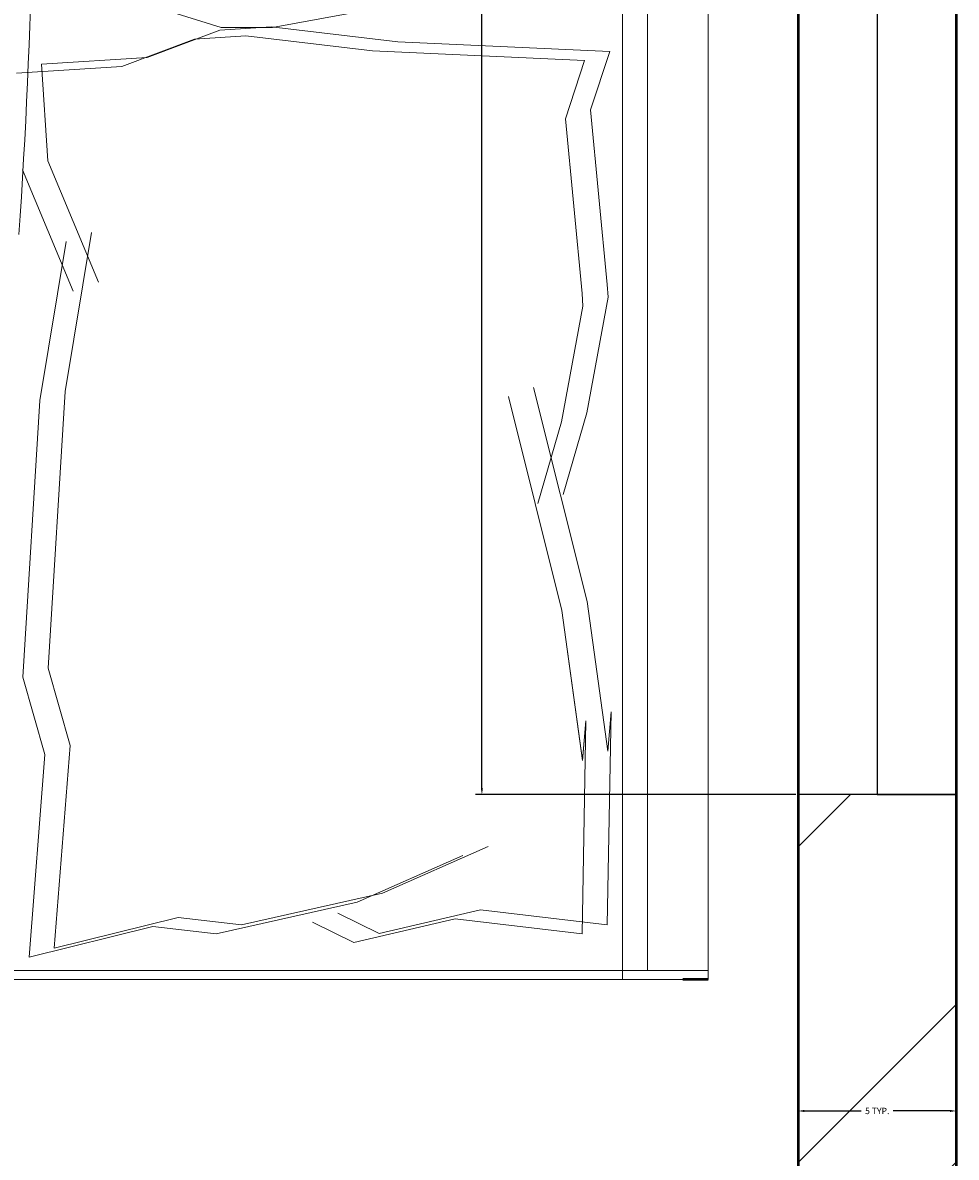
# Model space of a CAD drawing. Units: inches. Extents: x 1901 to 2863, y 888 to 2433.
# Tile 44 of 91: x 2726 to 2753, y 1563 to 1595. Entities that reach past the tile are written whole.
import ezdxf

# ---------------------------------------------------------------- set-up
doc = ezdxf.new("R2010")
doc.units = ezdxf.units.IN
for name, color, linetype, lineweight in [('A-ANNO-DIMS', 2, 'Continuous', 18), ('A-FURN', 8, 'Continuous', 18), ('A-GLAZ', 3, 'Continuous', 25), ('A-WALL', 7, 'Continuous', 50), ('A-WALL-PATT', 8, 'Continuous', 13)]:
    doc.layers.add(name, color=color, linetype=linetype, lineweight=lineweight)
doc.styles.get("Standard").update_dxf_attribs({"font": 'arial.ttf'})
doc.dimstyles.get("Standard").update_dxf_attribs({"dimtxt": 0.18, "dimasz": 0.18, "dimexe": 0.18, "dimexo": 0.0625, "dimgap": 0.09, "dimtad": 0, "dimtih": 1, "dimtoh": 1, "dimdec": 4, "dimzin": 0, "dimdsep": 46, "dimtxsty": 'Standard', "dimcen": 0.09, "dimadec": 0, "dimazin": 0, "dimtfac": 1, "dimtdec": 4, "dimtofl": 0, "dimtmove": 0, "dimatfit": 3, "dimfxl": 1, "dimtolj": 1, "dimtzin": 0, "dimarcsym": 0})

# ---------------------------------------------------------------- blocks, each defined once
blk = doc.blocks.new('BED-DOUBLE')
for p, q in [((0.026, 57.778), (0.026, 4.122)), ((0.744, 57.778), (30.62, 57.778)), ((0.744, 57.778), (30.62, 57.778)), ((18.633, 56.885), (15.109, 56.014)), ((18.633, 56.885), (15.109, 56.014)), ((19.351, 57.142), (15.827, 56.271)), ((19.351, 57.141), (15.827, 56.271)), ((18.18, 51.123), (18.633, 56.885)), ((18.18, 51.123), (18.633, 56.885)), ((18.898, 51.38), (19.351, 57.142)), ((18.898, 51.379), (19.351, 57.141)), ((7.22, 56.058), (10.106, 56.726)), ((7.22, 56.058), (10.106, 56.726)), ((10.106, 56.726), (11.28, 56.149)), ((10.106, 56.726), (11.28, 56.149)), ((2.897, 56.227), (2.788, 50.161)), ((2.897, 56.227), (2.788, 50.161)), ((2.897, 56.227), (6.502, 55.801)), ((2.897, 56.227), (6.502, 55.802)), ((3.615, 56.483), (3.506, 50.417)), ((3.615, 56.483), (3.506, 50.418)), ((3.615, 56.483), (7.22, 56.058)), ((3.615, 56.483), (7.22, 56.058)), ((6.502, 55.801), (9.388, 56.47)), ((6.502, 55.802), (9.388, 56.47)), ((13.307, 56.227), (9.297, 55.326)), ((13.307, 56.227), (9.297, 55.326)), ((9.388, 56.47), (10.563, 55.893)), ((9.388, 56.47), (10.563, 55.893)), ((14.025, 56.483), (10.015, 55.582)), ((14.025, 56.483), (10.015, 55.582)), ((15.109, 56.014), (13.307, 56.227)), ((15.109, 56.014), (13.307, 56.227)), ((15.827, 56.271), (14.025, 56.483)), ((15.827, 56.271), (14.025, 56.483)), ((10.015, 55.582), (7.007, 54.256)), ((10.015, 55.582), (7.007, 54.256)), ((9.297, 55.326), (6.289, 53.999)), ((9.297, 55.326), (6.289, 54)), ((3.506, 50.418), (3.598, 51.544)), ((3.506, 50.417), (3.598, 51.543)), ((3.598, 51.544), (4.19, 47.279)), ((3.598, 51.543), (4.19, 47.279)), ((19.523, 49.179), (18.898, 51.38)), ((19.523, 49.179), (18.898, 51.379)), ((2.788, 50.161), (2.881, 51.287)), ((2.788, 50.161), (2.881, 51.287)), ((2.881, 51.287), (3.472, 47.023)), ((2.881, 51.287), (3.472, 47.023)), ((18.806, 48.922), (18.18, 51.123)), ((18.806, 48.922), (18.18, 51.123)), ((19.039, 41.308), (19.523, 49.179)), ((19.039, 41.308), (19.523, 49.179)), ((18.322, 41.052), (18.806, 48.922)), ((18.322, 41.052), (18.806, 48.922)), ((4.19, 47.279), (5.709, 41.195)), ((4.19, 47.279), (5.709, 41.195)), ((3.472, 47.023), (4.991, 40.938)), ((3.472, 47.023), (4.991, 40.938)), ((4.869, 44.232), (4.2, 41.913)), ((4.869, 44.232), (4.2, 41.914)), ((4.151, 43.976), (3.482, 41.657)), ((4.151, 43.975), (3.482, 41.657)), ((3.482, 41.657), (2.875, 38.367)), ((3.482, 41.657), (2.875, 38.367)), ((4.2, 41.914), (3.593, 38.623)), ((4.2, 41.913), (3.593, 38.623)), ((17.573, 36.525), (18.322, 41.052)), ((17.573, 36.525), (18.322, 41.052)), ((18.291, 36.782), (19.039, 41.308)), ((18.291, 36.781), (19.039, 41.308)), ((3.593, 38.623), (3.615, 38.263)), ((3.593, 38.623), (3.615, 38.263)), ((2.875, 38.367), (2.897, 38.006)), ((2.875, 38.367), (2.897, 38.007)), ((3.615, 38.263), (4.088, 33.291)), ((3.615, 38.263), (4.088, 33.291)), ((19.538, 34.745), (18.096, 38.192)), ((19.538, 34.745), (18.096, 38.192)), ((2.897, 38.007), (3.371, 33.035)), ((2.897, 38.006), (3.371, 33.035)), ((18.82, 34.489), (17.378, 37.936)), ((18.82, 34.488), (17.378, 37.936)), ((18.993, 31.735), (18.82, 34.489)), ((18.993, 31.734), (18.82, 34.488)), ((4.088, 33.291), (3.542, 31.631)), ((4.088, 33.291), (3.542, 31.631)), ((3.371, 33.035), (2.824, 31.374)), ((3.371, 33.035), (2.824, 31.375)), ((16.706, 31.803), (19.71, 31.991)), ((16.706, 31.803), (19.71, 31.991)), ((14.64, 31.024), (16.706, 31.803)), ((14.64, 31.024), (16.706, 31.803)), ((15.988, 31.547), (18.993, 31.735)), ((15.988, 31.547), (18.993, 31.734)), ((2.824, 31.375), (8.859, 31.101)), ((2.824, 31.374), (8.859, 31.101)), ((3.542, 31.631), (9.577, 31.358)), ((3.542, 31.631), (9.577, 31.358)), ((9.577, 31.358), (13.182, 30.933)), ((9.577, 31.358), (13.182, 30.932)), ((13.922, 30.767), (15.988, 31.547)), ((13.922, 30.767), (15.988, 31.547)), ((8.859, 31.101), (12.464, 30.676)), ((8.859, 31.101), (12.464, 30.676)), ((13.182, 30.932), (14.64, 31.024)), ((13.182, 30.933), (14.64, 31.024)), ((8.85, 30.041), (12.422, 30.69)), ((8.85, 30.041), (12.422, 30.69)), ((12.422, 30.69), (13.883, 30.69)), ((12.422, 30.69), (13.883, 30.69)), ((12.464, 30.676), (13.922, 30.767)), ((12.464, 30.676), (13.922, 30.767)), ((13.883, 30.69), (15.993, 30.041)), ((13.883, 30.69), (15.993, 30.041))]:
    blk.add_line(p, q)
blk.add_arc((204.426, 23.944), 185.219, 176.08655, 186.78213)
blk.add_arc((204.426, 23.944), 185.219, 176.08655, 186.78213)
blk = doc.blocks.new('WIN-60')
for p, q in [((60, 2.25), (60, 4.5)), ((60, 4.5), (60, 0)), ((0, 2.25), (60, 2.25))]:
    blk.add_line(p, q)
blk = doc.blocks.new('*D19')
at = {"layer": 'A-ANNO-DIMS', "color": 0, "lineweight": -2, "transparency": 16777216}
for p, q in [((2748.364, 1633.499), (2739.246, 1633.499)), ((2739.426, 1633.319), (2739.426, 1603.682)), ((2739.426, 1573.679), (2739.426, 1603.316)), ((2748.364, 1573.499), (2739.246, 1573.499))]:
    blk.add_line(p, q, dxfattribs=at)
at = {"layer": 'A-ANNO-DIMS', "color": 0, "transparency": 16777216}
for points in [[(2739.396, 1633.319), (2739.456, 1633.319), (2739.426, 1633.499)], [(2739.396, 1573.679), (2739.456, 1573.679), (2739.426, 1573.499)]]:
    blk.add_solid(points, dxfattribs=at)
at = {"layer": 'Defpoints', "color": 0, "transparency": 16777216}
for p in [(2748.426, 1633.499), (2739.426, 1573.499), (2748.426, 1573.499)]:
    blk.add_point(p, dxfattribs=at)
at = {"layer": 'A-ANNO-DIMS', "color": 0, "transparency": 16777216, "insert": (2739.426, 1603.499), "char_height": 0.18, "attachment_point": 5}
blk.add_mtext('\\A1;WINDOW W1 60 TYP.', dxfattribs=at)
blk = doc.blocks.new('*D20')
at = {"layer": 'A-ANNO-DIMS', "color": 0, "lineweight": -2, "transparency": 16777216}
for p, q in [((2748.426, 1573.437), (2748.426, 1564.319)), ((2752.926, 1573.437), (2752.926, 1564.319)), ((2748.606, 1564.499), (2750.218, 1564.499)), ((2752.746, 1564.499), (2751.134, 1564.499))]:
    blk.add_line(p, q, dxfattribs=at)
at = {"layer": 'A-ANNO-DIMS', "color": 0, "transparency": 16777216}
for points in [[(2748.606, 1564.529), (2748.606, 1564.469), (2748.426, 1564.499)], [(2752.746, 1564.529), (2752.746, 1564.469), (2752.926, 1564.499)]]:
    blk.add_solid(points, dxfattribs=at)
at = {"layer": 'Defpoints', "color": 0, "transparency": 16777216}
for p in [(2748.426, 1573.499), (2752.926, 1573.499), (2752.926, 1564.499)]:
    blk.add_point(p, dxfattribs=at)
at = {"layer": 'A-ANNO-DIMS', "color": 0, "transparency": 16777216, "insert": (2750.676, 1564.499), "char_height": 0.18, "attachment_point": 5}
blk.add_mtext('\\A1;5 TYP.', dxfattribs=at)

msp = doc.modelspace()

# ---------------------------------------------------------------- hatches: boundary and pattern name
at = {"layer": 'A-WALL-PATT'}
h = msp.add_hatch(dxfattribs=at)
h.set_pattern_fill('ANSI32', color=256)
h.paths.add_polyline_path([(2443.926, 2139.888), (2439.426, 2139.888), (2439.426, 2069.348), (2441.676, 2069.348), (2443.926, 2069.348), (2443.926, 2078.634), (2521.926, 2078.634), (2521.926, 2075.067), (2524.176, 2075.067), (2526.426, 2075.067), (2526.426, 2078.634), (2571.755, 2078.634), (2571.755, 2080.884), (2571.755, 2083.134), (2443.926, 2083.134)])
h.paths.add_polyline_path([(2526.426, 2054.634), (2524.176, 2054.634), (2521.926, 2054.634), (2521.926, 2030.634), (2443.926, 2030.634), (2443.926, 2045.348), (2439.426, 2045.348), (2439.426, 1983.867), (2443.926, 1983.867), (2443.926, 2026.134), (2521.926, 2026.134), (2526.426, 2026.134)])
h.paths.add_polyline_path([(2443.926, 1923.867), (2439.426, 1923.867), (2439.426, 1872.634), (2443.926, 1872.634)])
h.paths.add_polyline_path([(2636.233, 1766.134), (2609.926, 1766.134), (2609.926, 1779.785), (2605.426, 1779.785), (2605.426, 1766.134), (2486.614, 1766.134), (2486.614, 1770.671), (2482.114, 1770.671), (2482.114, 1766.134), (2482.114, 1761.634), (2636.233, 1761.634), (2636.233, 1763.884)])
h.paths.add_polyline_path([(2519.536, 1663.384), (2519.536, 1665.634), (2494.926, 1665.634), (2481.831, 1665.634), (2481.831, 1663.384), (2481.831, 1661.134), (2490.426, 1661.134), (2490.426, 1640.157), (2494.926, 1640.157), (2494.926, 1661.134), (2519.536, 1661.134)])
h.paths.add_polyline_path([(2443.926, 1712.134), (2443.926, 1716.634), (2414.464, 1716.634), (2414.464, 1712.134), (2439.426, 1712.134), (2439.426, 1545.507), (2443.926, 1545.507), (2443.926, 1661.134), (2448.475, 1661.134), (2448.475, 1665.634), (2443.926, 1665.634)])
h.paths.add_polyline_path([(2343.426, 1712.134), (2365.525, 1712.134), (2365.525, 1714.384), (2365.525, 1716.634), (2333.871, 1716.634), (2333.871, 1714.384), (2333.871, 1712.134), (2338.926, 1712.134), (2338.926, 1575.634), (2338.926, 1545.507), (2343.426, 1545.507), (2343.426, 1547.507), (2343.426, 1580.134)])
h.paths.add_polyline_path([(2752.926, 1665.634), (2579.536, 1665.634), (2579.536, 1661.134), (2615.926, 1661.134), (2615.926, 1529.134), (2598.931, 1529.134), (2598.931, 1524.634), (2623.127, 1524.634), (2623.127, 1526.884), (2623.127, 1529.134), (2620.426, 1529.134), (2620.426, 1661.134), (2748.426, 1661.134), (2748.426, 1633.499), (2752.926, 1633.499)])
h.paths.add_polyline_path([(2752.926, 1419.929), (2748.426, 1419.929), (2748.426, 1400.134), (2659.426, 1400.134), (2659.426, 1444.333), (2657.176, 1444.333), (2654.926, 1444.333), (2654.926, 1400.134), (2643.649, 1400.134), (2643.649, 1395.634), (2748.426, 1395.634), (2748.426, 1364.035), (2752.926, 1364.035)])
h.paths.add_polyline_path([(2752.926, 1492.878), (2748.426, 1492.878), (2748.426, 1476.634), (2667.426, 1476.634), (2667.426, 1479.71), (2665.176, 1479.71), (2662.926, 1479.71), (2662.926, 1476.634), (2654.926, 1476.634), (2654.926, 1469.536), (2659.426, 1469.536), (2659.426, 1472.134), (2748.426, 1472.134), (2748.426, 1455.929), (2752.926, 1455.929)])
h.paths.add_polyline_path([(2752.926, 1304.035), (2748.426, 1304.035), (2748.426, 1263.634), (2738.66, 1263.634), (2738.66, 1259.134), (2752.926, 1259.134)])
h.paths.add_polyline_path([(2685.926, 1259.134), (2695.49, 1259.134), (2695.49, 1261.384), (2695.49, 1263.634), (2677.837, 1263.634), (2677.837, 1261.384), (2677.837, 1259.134), (2681.426, 1259.134), (2681.426, 1203.634), (2653.277, 1203.634), (2653.277, 1199.134), (2685.926, 1199.134), (2685.926, 1203.634)])
h.paths.add_polyline_path([(2609.426, 1395.634), (2611.848, 1395.634), (2611.848, 1400.134), (2598.888, 1400.134), (2598.888, 1397.884), (2598.888, 1395.634), (2604.926, 1395.634), (2604.926, 1268.134), (2554.726, 1268.134), (2554.726, 1265.884), (2554.726, 1263.634), (2604.926, 1263.634), (2604.926, 1203.634), (2571.306, 1203.634), (2571.306, 1199.134), (2604.926, 1199.134), (2629.277, 1199.134), (2629.277, 1201.384), (2629.277, 1203.634), (2609.426, 1203.634), (2609.426, 1258.634), (2609.426, 1259.134), (2654.804, 1259.134), (2654.804, 1263.634), (2609.426, 1263.634)])
h.paths.add_polyline_path([(2443.926, 1304.035), (2439.426, 1304.035), (2439.426, 1259.134), (2443.926, 1259.134), (2456.16, 1259.134), (2456.16, 1261.384), (2456.16, 1263.634), (2443.926, 1263.634)])
h.paths.add_polyline_path([(2525.426, 1263.634), (2531.778, 1263.634), (2531.778, 1268.134), (2520.926, 1268.134), (2520.926, 1263.634), (2511.409, 1263.634), (2511.409, 1259.134), (2520.926, 1259.134), (2520.926, 1199.134), (2547.306, 1199.134), (2547.306, 1201.384), (2547.306, 1203.634), (2525.426, 1203.634)])
h.paths.add_polyline_path([(2443.926, 1434.842), (2439.426, 1434.842), (2439.426, 1364.035), (2441.676, 1364.035), (2443.926, 1364.035)])
h.paths.add_polyline_path([(2567.134, 1400.134), (2443.926, 1400.134), (2443.926, 1395.634), (2567.134, 1395.634)])
h.paths.add_polyline_path([(2443.926, 1545.507), (2439.426, 1545.507), (2439.426, 1494.842), (2443.926, 1494.842)])
h.paths.add_polyline_path([(2494.926, 1553.349), (2492.676, 1553.349), (2490.426, 1553.349), (2490.426, 1524.634), (2494.926, 1524.634), (2525.936, 1524.634), (2525.936, 1526.884), (2525.936, 1529.134), (2494.926, 1529.134)])
h.paths.add_polyline_path([(2752.926, 1573.499), (2748.426, 1573.499), (2748.426, 1529.134), (2657.759, 1529.134), (2657.759, 1524.634), (2662.926, 1524.634), (2662.926, 1498.631), (2667.426, 1498.631), (2667.426, 1524.634), (2748.426, 1524.634), (2748.426, 1516.878), (2752.926, 1516.878)])
h.paths.add_polyline_path([(2038.602, 2237.418), (2080.174, 2237.418), (2080.174, 2256.075), (2038.602, 2256.075)], flags=9)
h.paths.add_polyline_path([(2292.009, 1062.394), (2539.932, 1062.394), (2539.932, 1099.487), (2292.009, 1099.487)], flags=9)
h.paths.add_polyline_path([(2424.91, 1832.253), (2448.513, 1832.253), (2448.513, 1846.678), (2424.91, 1846.678)], flags=9)
h.paths.add_polyline_path([(2359.076, 1832.253), (2382.678, 1832.253), (2382.678, 1846.678), (2359.076, 1846.678)], flags=9)
h.paths.add_polyline_path([(2352.899, 1684.802), (2367.543, 1684.802), (2367.543, 1697.167), (2352.899, 1697.167)], flags=9)
h.paths.add_polyline_path([(2079.288, 1755.826), (2169.024, 1755.826), (2169.024, 1774.372), (2079.288, 1774.372)], flags=9)
h.paths.add_polyline_path([(2404.09, 1373.857), (2404.09, 1463.593), (2385.544, 1463.593), (2385.544, 1373.857)], flags=9)
h.paths.add_polyline_path([(2268.091, 2236.371), (2309.636, 2236.371), (2309.636, 2255.028), (2268.091, 2255.028)], flags=9)
h.paths.add_polyline_path([(2575.96, 1700.951), (2665.696, 1700.951), (2665.696, 1719.498), (2575.96, 1719.498)], flags=9)
h.paths.add_polyline_path([(2302.962, 1878.474), (2329.524, 1878.474), (2329.524, 1888.777), (2302.962, 1888.777)], flags=9)
h.paths.add_polyline_path([(2097.415, 2240.576), (2126.573, 2240.576), (2126.573, 2259.233), (2097.415, 2259.233)], flags=9)
h.paths.add_polyline_path([(2208.725, 2246.124), (2237.882, 2246.124), (2237.882, 2264.781), (2208.725, 2264.781)], flags=9)
h.paths.add_polyline_path([(2038.147, 1925.958), (2076.987, 1925.958), (2076.987, 1944.615), (2038.147, 1944.615)], flags=9)
h.paths.add_polyline_path([(2239.144, 1926.672), (2288.465, 1926.672), (2288.465, 1945.329), (2239.144, 1945.329)], flags=9)
h.paths.add_polyline_path([(2175.429, 2007.33), (2212.356, 2007.33), (2212.356, 2025.987), (2175.429, 2025.987)], flags=9)
h.paths.add_polyline_path([(2225.034, 2091.794), (2263.875, 2091.794), (2263.875, 2110.451), (2225.034, 2110.451)], flags=9)
h.paths.add_polyline_path([(2035.398, 2098.478), (2074.238, 2098.478), (2074.238, 2117.135), (2035.398, 2117.135)], flags=9)
h.paths.add_polyline_path([(2050.102, 2029.209), (2083.26, 2029.209), (2083.26, 2047.866), (2050.102, 2047.866)], flags=9)
h.paths.add_polyline_path([(2069.677, 1956.719), (2098.835, 1956.719), (2098.835, 1975.376), (2069.677, 1975.376)], flags=9)
h.paths.add_polyline_path([(2328.62, 1753.336), (2361.663, 1753.336), (2361.663, 1771.993), (2328.62, 1771.993)], flags=9)
h.paths.add_polyline_path([(2395.162, 2060.888), (2395.162, 2140.654), (2378.676, 2140.654), (2378.676, 2060.888)], flags=9)
h.paths.add_polyline_path([(2463.728, 2059.02), (2492.886, 2059.02), (2492.886, 2077.677), (2463.728, 2077.677)], flags=9)
h.paths.add_polyline_path([(2458.027, 2181.536), (2496.868, 2181.536), (2496.868, 2200.194), (2458.027, 2200.194)], flags=9)
h.paths.add_polyline_path([(2456.855, 2228.831), (2498.401, 2228.831), (2498.401, 2247.488), (2456.855, 2247.488)], flags=9)
h.paths.add_polyline_path([(2527.577, 2243.074), (2556.735, 2243.074), (2556.735, 2261.731), (2527.577, 2261.731)], flags=9)
h.paths.add_polyline_path([(2694.461, 2232.767), (2736.033, 2232.767), (2736.033, 2251.425), (2694.461, 2251.425)], flags=9)
h.paths.add_polyline_path([(2637.821, 2249.225), (2666.979, 2249.225), (2666.979, 2267.882), (2637.821, 2267.882)], flags=9)
h.paths.add_polyline_path([(2623.687, 2183.541), (2662.528, 2183.541), (2662.528, 2202.199), (2623.687, 2202.199)], flags=9)
h.paths.add_polyline_path([(2691.965, 2021.5), (2725.124, 2021.5), (2725.124, 2040.157), (2691.965, 2040.157)], flags=9)
h.paths.add_polyline_path([(2621.043, 1975.912), (2662.335, 1975.912), (2662.335, 1994.569), (2621.043, 1994.569)], flags=9)
h.paths.add_polyline_path([(2479.032, 1927.62), (2519.844, 1927.62), (2519.844, 1946.277), (2479.032, 1946.277)], flags=9)
h.paths.add_polyline_path([(2670.941, 1849.076), (2716.005, 1849.076), (2716.005, 1867.734), (2670.941, 1867.734)], flags=9)
h.paths.add_polyline_path([(2523.613, 1782.956), (2550.175, 1782.956), (2550.175, 1793.26), (2523.613, 1793.26)], flags=9)
h.paths.add_polyline_path([(2450.841, 1207.331), (2492.386, 1207.331), (2492.386, 1225.989), (2450.841, 1225.989)], flags=9)
h.paths.add_polyline_path([(2527.751, 1203.841), (2556.908, 1203.841), (2556.908, 1222.499), (2527.751, 1222.499)], flags=9)
h.paths.add_polyline_path([(2639.111, 1207.2), (2668.268, 1207.2), (2668.268, 1225.857), (2639.111, 1225.857)], flags=9)
h.paths.add_polyline_path([(2692.594, 1218.965), (2734.167, 1218.965), (2734.167, 1237.623), (2692.594, 1237.623)], flags=9)
h.paths.add_polyline_path([(2669.266, 1366.329), (2708.106, 1366.329), (2708.106, 1384.987), (2669.266, 1384.987)], flags=25)
h.paths.add_polyline_path([(2463.313, 1358.031), (2502.153, 1358.031), (2502.153, 1376.688), (2463.313, 1376.688)], flags=9)
h.paths.add_polyline_path([(2494.725, 1449.963), (2531.652, 1449.963), (2531.652, 1468.62), (2494.725, 1468.62)], flags=9)
h.paths.add_polyline_path([(2675.565, 1422.157), (2708.724, 1422.157), (2708.724, 1440.815), (2675.565, 1440.815)], flags=25)
h.paths.add_polyline_path([(2685.634, 1493.891), (2714.792, 1493.891), (2714.792, 1512.548), (2685.634, 1512.548)], flags=9)
h.paths.add_polyline_path([(2686.805, 1529.913), (2725.645, 1529.913), (2725.645, 1548.57), (2686.805, 1548.57)], flags=25)
h.paths.add_polyline_path([(2503.651, 1537.991), (2552.972, 1537.991), (2552.972, 1556.648), (2503.651, 1556.648)], flags=9)
h.paths.add_polyline_path([(2291.713, 1643.504), (2318.275, 1643.504), (2318.275, 1653.807), (2291.713, 1653.807)], flags=9)
h.paths.add_polyline_path([(2450.626, 1610.52), (2477.189, 1610.52), (2477.189, 1620.824), (2450.626, 1620.824)], flags=9)
h.paths.add_polyline_path([(2359.985, 1551.814), (2422.253, 1551.814), (2422.253, 1562.117), (2359.985, 1562.117)], flags=9)
h.paths.add_polyline_path([(2280.106, 1249.006), (2321.651, 1249.006), (2321.651, 1267.663), (2280.106, 1267.663)], flags=9)
h.paths.add_polyline_path([(2164.057, 1274.232), (2193.215, 1274.232), (2193.215, 1292.889), (2164.057, 1292.889)], flags=9)
h.paths.add_polyline_path([(2118.21, 1277.694), (2151.252, 1277.694), (2151.252, 1296.351), (2118.21, 1296.351)], flags=9)
h.paths.add_polyline_path([(2031.946, 1268.529), (2073.519, 1268.529), (2073.519, 1287.187), (2031.946, 1287.187)], flags=9)
h.paths.add_polyline_path([(2050.199, 1409.079), (2089.04, 1409.079), (2089.04, 1427.736), (2050.199, 1427.736)], flags=9)
h.paths.add_polyline_path([(2243.743, 1421.032), (2282.584, 1421.032), (2282.584, 1439.689), (2243.743, 1439.689)], flags=9)
h.paths.add_polyline_path([(2190.746, 1509.769), (2231.558, 1509.769), (2231.558, 1528.426), (2190.746, 1528.426)], flags=9)
h.paths.add_polyline_path([(2058.392, 1475.415), (2091.55, 1475.415), (2091.55, 1494.073), (2058.392, 1494.073)], flags=9)
h.paths.add_polyline_path([(2062.447, 1553.09), (2091.605, 1553.09), (2091.605, 1571.747), (2062.447, 1571.747)], flags=9)
h.paths.add_polyline_path([(2219.524, 1590.365), (2266.147, 1590.365), (2266.147, 1609.022), (2219.524, 1609.022)], flags=9)
h.paths.add_polyline_path([(2041.072, 1584.188), (2079.912, 1584.188), (2079.912, 1602.845), (2041.072, 1602.845)], flags=9)

# ---------------------------------------------------------------- linework, layer by layer
at = {"layer": 'A-FURN'}
for p, q in [((2744.142, 1622.154), (2744.142, 1568.498)), ((2744.142, 1622.154), (2744.142, 1568.498)), ((2743.424, 1621.898), (2743.424, 1568.241)), ((2743.424, 1621.898), (2743.424, 1568.241)), ((2745.864, 1568.498), (2715.987, 1568.498)), ((2745.864, 1568.498), (2715.987, 1568.498))]:
    msp.add_line(p, q, dxfattribs=at)
at = {"layer": 'A-WALL'}
for p, q in [((2752.926, 1665.634), (2752.926, 1259.134)), ((2748.426, 1661.134), (2748.426, 1529.134)), ((2745.864, 1568.241), (2745.146, 1568.241))]:
    msp.add_line(p, q, dxfattribs=at)

# ---------------------------------------------------------------- block references
at = {"layer": 'A-FURN', "rotation": 180}
msp.add_blockref('BED-DOUBLE', (2745.89, 1626.019), dxfattribs=at)
at = {"layer": 'A-GLAZ', "rotation": 270.0000000000013}
msp.add_blockref('WIN-60', (2748.426, 1633.5), dxfattribs=at)

# ---------------------------------------------------------------- dimensions: what is measured, and where the dimension line sits
at = {"layer": 'A-ANNO-DIMS'}
dim = msp.add_linear_dim(base=(2739.426, 1573.499), p1=(2748.426, 1633.499), p2=(2748.426, 1573.499), angle=270, text='WINDOW W1 <> TYP.', dimstyle='Standard', override={"dimdec": 0, "dimlfac": 1, "dimrnd": 0, "dimzin": 0, "dimdsep": 46, "dimlunit": 2}, dxfattribs=at)
dim.commit()
dim.dimension.update_dxf_attribs({"geometry": '*D19', "text_midpoint": (2739.426, 1603.499)})
dim = msp.add_linear_dim(base=(2752.926174575, 1564.499050932), p1=(2748.426174575, 1573.499050932), p2=(2752.926174575, 1573.499050932), text='<> TYP.', dimstyle='Standard', override={"dimdec": 0, "dimlfac": 1, "dimrnd": 0, "dimzin": 0, "dimdsep": 46, "dimlunit": 2}, dxfattribs=at)
dim.commit()
dim.dimension.update_dxf_attribs({"geometry": '*D20', "text_midpoint": (2750.676174575, 1564.499050932)})

doc.saveas('drawing.dxf')
